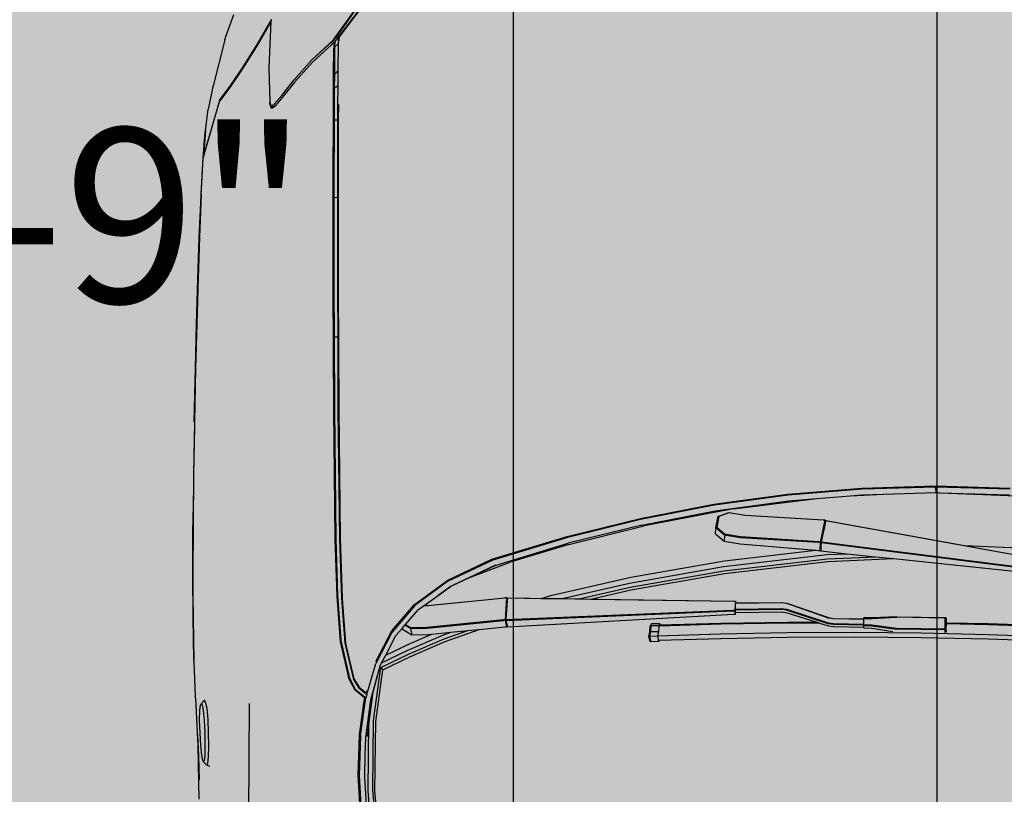
# Model space of a CAD drawing. Units: inches. Extents: x 1884 to 2398, y 474 to 1488.
# Tile 15 of 39: x 2186 to 2233, y 699 to 736. Entities that reach past the tile are written whole.
import ezdxf

# ---------------------------------------------------------------- set-up
doc = ezdxf.new("R2010")
doc.units = ezdxf.units.IN
doc.header["$MEASUREMENT"] = 0
doc.layers.get('0').update_dxf_attribs({"color": 250})
for name, color, linetype, lineweight in [('A-ANNO-DIMS', 2, 'Continuous', 18), ('A-AREA-IDEN', 7, 'Continuous', 18), ('C-VEHI', 8, 'Continuous', 18)]:
    doc.layers.add(name, color=color, linetype=linetype, lineweight=lineweight)
doc.layers.add('Edges', color=250, linetype='Continuous')
doc.layers.add('L-PVMT-PATT', color=9, linetype='Continuous', lineweight=13, true_color=0xc7c8ca)
doc.styles.get("Standard").update_dxf_attribs({"font": 'arial.ttf'})
doc.dimstyles.get("Standard").update_dxf_attribs({"dimtxt": 7, "dimasz": 0.18, "dimexe": 0.18, "dimexo": 0.0625, "dimgap": 0.09, "dimtad": 0, "dimtih": 1, "dimtoh": 1, "dimzin": 0, "dimdsep": 46, "dimlunit": 3, "dimtxsty": 'Standard', "dimcen": 0.09, "dimadec": 0, "dimazin": 0, "dimtfac": 1, "dimtofl": 0, "dimtmove": 0, "dimatfit": 3, "dimfxl": 1, "dimtolj": 1, "dimtzin": 0, "dimarcsym": 0})

# ---------------------------------------------------------------- blocks, each defined once
blk = doc.blocks.new('Nissan Qashqai pl')
at = {"layer": 'Edges'}
for p, q in [((8.4387, 12.0674), (8.4359, 11.9861)), ((8.4397, 12.0674), (8.4369, 11.9861)), ((8.4517, 12.0674), (8.4489, 11.9858)), ((8.4541, 11.9857), (8.4568, 12.0669)), ((8.3406, 11.9567), (8.3448, 12.0536)), ((8.3575, 12.0475), (8.3104, 11.7881)), ((8.336, 11.7828), (8.3688, 12.0419)), ((8.3702, 12.0427), (8.3374, 11.7826)), ((8.3565, 11.8707), (8.3746, 12.0435)), ((8.2765, 11.9273), (8.2804, 12.0305)), ((8.2682, 11.9221), (8.2708, 12.0123)), ((8.2719, 12.0118), (8.2695, 11.9221)), ((8.2765, 11.9273), (8.2788, 12.0114)), ((8.3406, 11.9567), (8.3495, 12.0053)), ((8.4359, 11.9861), (8.4348, 11.9346)), ((8.4369, 11.9861), (8.4358, 11.9346)), ((8.4489, 11.9858), (8.4471, 11.9043)), ((8.4523, 11.9043), (8.4541, 11.9857)), ((8.31, 11.7882), (8.3406, 11.9567)), ((8.4272, 11.8746), (8.4281, 11.9336)), ((8.4287, 11.9335), (8.4278, 11.8745)), ((8.4281, 11.9336), (8.429, 11.9345)), ((8.4281, 11.9336), (8.4287, 11.9336)), ((8.4287, 11.9335), (8.4281, 11.9336)), ((8.429, 11.9345), (8.4287, 11.9336)), ((8.4287, 11.9336), (8.4287, 11.9335)), ((8.4418, 11.9332), (8.4287, 11.9335)), ((8.4328, 11.9347), (8.429, 11.9345)), ((8.429, 11.9345), (8.4326, 11.9345)), ((8.4328, 11.9347), (8.4326, 11.9345)), ((8.4326, 11.9345), (8.4348, 11.9344)), ((8.4348, 11.9346), (8.4328, 11.9347)), ((8.4348, 11.9346), (8.4348, 11.9344)), ((8.4358, 11.9346), (8.4348, 11.9346)), ((8.4348, 11.9344), (8.4358, 11.9344)), ((8.4358, 11.9346), (8.4358, 11.9344)), ((8.4459, 11.9344), (8.4358, 11.9346)), ((8.4358, 11.9344), (8.4422, 11.9342)), ((8.441, 11.8742), (8.4418, 11.9332)), ((8.4418, 11.9332), (8.4422, 11.9342)), ((8.4431, 11.9332), (8.4418, 11.9332)), ((8.4422, 11.9342), (8.4459, 11.9344)), ((8.4422, 11.9342), (8.4431, 11.9332)), ((8.4431, 11.9332), (8.4422, 11.8742)), ((8.4464, 11.9334), (8.4431, 11.9332)), ((8.4459, 11.9344), (8.4459, 11.9344)), ((8.2708, 11.8319), (8.2682, 11.9221)), ((8.2763, 11.9223), (8.2695, 11.9221)), ((8.2695, 11.9221), (8.2763, 11.9219)), ((8.2695, 11.9221), (8.2719, 11.8323)), ((8.2763, 11.9223), (8.2764, 11.9263)), ((8.2763, 11.9219), (8.2763, 11.9223)), ((8.2781, 11.8585), (8.2763, 11.9219)), ((8.2764, 11.9263), (8.2765, 11.9273)), ((8.4471, 11.9043), (8.4464, 11.8227)), ((8.4516, 11.823), (8.4523, 11.9043)), ((8.3542, 11.8485), (8.3565, 11.8707)), ((8.3599, 11.7906), (8.3565, 11.8707)), ((8.4272, 11.8746), (8.4286, 11.8445)), ((8.4292, 11.8445), (8.4278, 11.8745)), ((8.4368, 11.8443), (8.441, 11.8742)), ((8.438, 11.8443), (8.4422, 11.8742)), ((8.4408, 11.8444), (8.4452, 11.8698)), ((8.28, 11.818), (8.2781, 11.8585)), ((8.2788, 11.8327), (8.2781, 11.8585)), ((8.2789, 11.8319), (8.2781, 11.8585)), ((8.3505, 11.8139), (8.3542, 11.8485)), ((8.3567, 11.7903), (8.3542, 11.8485)), ((8.4286, 11.8445), (8.4285, 11.8345)), ((8.4291, 11.8345), (8.4292, 11.8445)), ((8.4366, 11.8345), (8.4368, 11.8443)), ((8.4379, 11.8345), (8.438, 11.8443)), ((8.4406, 11.8344), (8.4408, 11.8444)), ((8.2781, 11.7423), (8.2708, 11.8319)), ((8.2719, 11.8323), (8.2793, 11.7426)), ((8.2789, 11.8319), (8.2788, 11.8327)), ((8.28, 11.818), (8.2789, 11.8319)), ((8.4291, 11.8345), (8.4285, 11.8345)), ((8.4298, 11.8345), (8.4291, 11.8345)), ((8.4292, 11.7978), (8.4298, 11.8345)), ((8.4304, 11.8345), (8.4298, 11.7978)), ((8.4304, 11.8345), (8.4298, 11.8345)), ((8.436, 11.8344), (8.4304, 11.8345)), ((8.4355, 11.7977), (8.436, 11.8344)), ((8.4366, 11.8343), (8.436, 11.8344)), ((8.4366, 11.8345), (8.4379, 11.8345)), ((8.4366, 11.8344), (8.4366, 11.8345)), ((8.4373, 11.8344), (8.4366, 11.8344)), ((8.4373, 11.8344), (8.4366, 11.8343)), ((8.4366, 11.8343), (8.4366, 11.8344)), ((8.4373, 11.8344), (8.4367, 11.7977)), ((8.4379, 11.8344), (8.4373, 11.8344)), ((8.4379, 11.8343), (8.4373, 11.8344)), ((8.4379, 11.8344), (8.4379, 11.8345)), ((8.4397, 11.8344), (8.4379, 11.8343)), ((8.4379, 11.8343), (8.4379, 11.8344)), ((8.4391, 11.7978), (8.4397, 11.8344)), ((8.4406, 11.8344), (8.4397, 11.8344)), ((8.452, 11.7418), (8.4516, 11.823)), ((8.2834, 11.7773), (8.28, 11.818)), ((8.3472, 11.7821), (8.3505, 11.8139)), ((8.3516, 11.79), (8.3505, 11.8139)), ((8.4464, 11.8227), (8.4468, 11.7413)), ((8.3092, 11.7863), (8.3093, 11.7873)), ((8.3093, 11.7873), (8.3367, 11.7816)), ((8.3159, 11.7869), (8.3093, 11.7873)), ((8.31, 11.7882), (8.3104, 11.7881)), ((8.3104, 11.7881), (8.3159, 11.7869)), ((8.3159, 11.7869), (8.336, 11.7828)), ((8.3662, 11.6639), (8.3516, 11.79)), ((8.3713, 11.6645), (8.3567, 11.7903)), ((8.3745, 11.665), (8.3599, 11.7906)), ((8.4107, 11.7411), (8.4281, 11.7914)), ((8.4287, 11.7914), (8.4111, 11.741)), ((8.4179, 11.7406), (8.4344, 11.7912)), ((8.4357, 11.7912), (8.4193, 11.7407)), ((8.4281, 11.7914), (8.4292, 11.7978)), ((8.4298, 11.7978), (8.4287, 11.7914)), ((8.4344, 11.7912), (8.4355, 11.7977)), ((8.4347, 11.7805), (8.4381, 11.7914)), ((8.4367, 11.7977), (8.4357, 11.7912)), ((8.4381, 11.7914), (8.4391, 11.7978)), ((8.296, 11.6762), (8.2834, 11.7773)), ((8.2862, 11.7434), (8.2834, 11.7773)), ((8.3038, 11.6903), (8.3095, 11.7853)), ((8.3099, 11.7851), (8.3042, 11.6901)), ((8.3092, 11.7863), (8.3099, 11.7851)), ((8.3095, 11.7853), (8.3092, 11.7863)), ((8.3298, 11.6848), (8.3355, 11.7798)), ((8.3369, 11.7796), (8.3312, 11.6846)), ((8.3355, 11.7798), (8.3366, 11.7806)), ((8.336, 11.7828), (8.3374, 11.7826)), ((8.3367, 11.7816), (8.3366, 11.7806)), ((8.3366, 11.7806), (8.3369, 11.7796)), ((8.3367, 11.7816), (8.347, 11.7811)), ((8.3374, 11.7826), (8.3406, 11.7824)), ((8.3385, 11.6842), (8.3464, 11.7761)), ((8.3458, 11.7813), (8.3406, 11.7824)), ((8.3406, 11.7824), (8.3457, 11.7821)), ((8.3458, 11.7813), (8.3457, 11.7821)), ((8.3457, 11.7821), (8.3472, 11.7821)), ((8.347, 11.7811), (8.3458, 11.7813)), ((8.3464, 11.7761), (8.3467, 11.7791)), ((8.3593, 11.6651), (8.3464, 11.7761)), ((8.3467, 11.7791), (8.347, 11.7811)), ((8.4222, 11.7413), (8.4337, 11.7775)), ((8.4337, 11.7775), (8.4347, 11.7805)), ((8.4337, 11.7775), (8.4339, 11.7423)), ((8.4347, 11.7805), (8.4348, 11.7421)), ((8.2905, 11.6524), (8.2781, 11.7423)), ((8.2793, 11.7426), (8.2916, 11.6528)), ((8.2985, 11.654), (8.2862, 11.7434)), ((8.4097, 11.7348), (8.4107, 11.7411)), ((8.4111, 11.741), (8.41, 11.7346)), ((8.417, 11.7342), (8.4179, 11.7406)), ((8.4193, 11.7407), (8.4183, 11.7343)), ((8.4213, 11.735), (8.4222, 11.7413)), ((8.4339, 11.7423), (8.4353, 11.6613)), ((8.4348, 11.7421), (8.4362, 11.661)), ((8.4468, 11.7413), (8.4482, 11.66)), ((8.4534, 11.6608), (8.452, 11.7418)), ((8.4104, 11.6791), (8.4097, 11.7348)), ((8.41, 11.7346), (8.4108, 11.6791)), ((8.4177, 11.678), (8.417, 11.7342)), ((8.4183, 11.7343), (8.4191, 11.678)), ((8.4221, 11.6787), (8.4213, 11.735)), ((8.3005, 11.6706), (8.3038, 11.6903)), ((8.3042, 11.6901), (8.3009, 11.6704)), ((8.3264, 11.6652), (8.3298, 11.6848)), ((8.3312, 11.6846), (8.3278, 11.665)), ((8.3352, 11.6646), (8.3385, 11.6842)), ((8.296, 11.6762), (8.3166, 11.5675)), ((8.3053, 11.6574), (8.3005, 11.6706)), ((8.3009, 11.6704), (8.3054, 11.6583)), ((8.4086, 11.6764), (8.4045, 11.4011)), ((8.4056, 11.5028), (8.4082, 11.6766)), ((8.4082, 11.6785), (8.4104, 11.6791)), ((8.4082, 11.6785), (8.4086, 11.6784)), ((8.4082, 11.6766), (8.4082, 11.6785)), ((8.4086, 11.6784), (8.4086, 11.6764)), ((8.4086, 11.6784), (8.4117, 11.6782)), ((8.4104, 11.6791), (8.4108, 11.6791)), ((8.4104, 11.6786), (8.4104, 11.6791)), ((8.4108, 11.6786), (8.4104, 11.6786)), ((8.4104, 11.6786), (8.4108, 11.6784)), ((8.4108, 11.6791), (8.4108, 11.6786)), ((8.4108, 11.6786), (8.4108, 11.6784)), ((8.4108, 11.6784), (8.4117, 11.6783)), ((8.4117, 11.6783), (8.4117, 11.6782)), ((8.4117, 11.6783), (8.4177, 11.678)), ((8.4117, 11.6782), (8.419, 11.6778)), ((8.4177, 11.678), (8.4191, 11.678)), ((8.419, 11.6778), (8.4203, 11.6778)), ((8.419, 11.6758), (8.419, 11.6778)), ((8.4305, 11.3996), (8.419, 11.6758)), ((8.4191, 11.678), (8.4221, 11.6787)), ((8.4238, 11.6786), (8.4203, 11.6778)), ((8.4203, 11.6778), (8.4204, 11.6758)), ((8.4204, 11.6758), (8.4319, 11.3996)), ((8.4238, 11.6786), (8.4221, 11.6787)), ((8.4238, 11.6766), (8.4238, 11.6786)), ((8.4394, 11.4014), (8.4238, 11.6766)), ((8.3054, 11.6583), (8.3053, 11.6574)), ((8.319, 11.6546), (8.3053, 11.6574)), ((8.3054, 11.6583), (8.3182, 11.6557)), ((8.3182, 11.6557), (8.3264, 11.6652)), ((8.319, 11.6546), (8.3182, 11.6557)), ((8.3278, 11.665), (8.319, 11.6546)), ((8.3264, 11.6542), (8.3352, 11.6646)), ((8.3278, 11.665), (8.3352, 11.6646)), ((8.3792, 11.5515), (8.3593, 11.6651)), ((8.3864, 11.5497), (8.3662, 11.6639)), ((8.3913, 11.5506), (8.3713, 11.6645)), ((8.3945, 11.5513), (8.3745, 11.665)), ((8.4353, 11.6613), (8.4375, 11.5863)), ((8.4362, 11.661), (8.4385, 11.5858)), ((8.4482, 11.66), (8.4505, 11.5843)), ((8.4557, 11.5855), (8.4534, 11.6608)), ((8.3076, 11.5631), (8.2905, 11.6524)), ((8.2916, 11.6528), (8.3089, 11.5631)), ((8.3157, 11.5647), (8.2985, 11.654)), ((8.3264, 11.6542), (8.319, 11.6546)), ((8.4377, 11.5857), (8.4357, 11.5864)), ((8.4357, 11.5864), (8.4359, 11.5765)), ((8.4357, 11.5864), (8.4375, 11.5863)), ((8.4375, 11.5863), (8.4375, 11.5862)), ((8.4379, 11.5758), (8.4377, 11.5857)), ((8.445, 11.5853), (8.4377, 11.5857)), ((8.4452, 11.5754), (8.445, 11.5853)), ((8.4503, 11.5841), (8.445, 11.5853)), ((8.4572, 11.5854), (8.4503, 11.5841)), ((8.4505, 11.5742), (8.4503, 11.5841)), ((8.4557, 11.5855), (8.4572, 11.5854)), ((8.4557, 11.5853), (8.4557, 11.5855)), ((8.4572, 11.5854), (8.4574, 11.5755)), ((8.4359, 11.5765), (8.4379, 11.5758)), ((8.4359, 11.5765), (8.4377, 11.5753)), ((8.4387, 11.5749), (8.4377, 11.5753)), ((8.4379, 11.5758), (8.4452, 11.5754)), ((8.4384, 11.5752), (8.4457, 11.5749)), ((8.446, 11.5746), (8.4387, 11.5749)), ((8.4452, 11.5754), (8.4505, 11.5742)), ((8.4507, 11.5734), (8.446, 11.5746)), ((8.4505, 11.5742), (8.4574, 11.5755)), ((8.4507, 11.5734), (8.4505, 11.5742)), ((8.4559, 11.5744), (8.4507, 11.5734)), ((8.4574, 11.5755), (8.4559, 11.5744)), ((8.3296, 11.4739), (8.3076, 11.5631)), ((8.3089, 11.5631), (8.3311, 11.4733)), ((8.3157, 11.5647), (8.3377, 11.4753)), ((8.3392, 11.4758), (8.3166, 11.5675)), ((8.4009, 11.4559), (8.3792, 11.5515)), ((8.4051, 11.4678), (8.3864, 11.5497)), ((8.4054, 11.4887), (8.3913, 11.5506)), ((8.4056, 11.5028), (8.3945, 11.5513)), ((8.4054, 11.4887), (8.4056, 11.5028)), ((8.4051, 11.4678), (8.4054, 11.4887)), ((8.3392, 11.4758), (8.3608, 11.4048)), ((8.3573, 11.3824), (8.3296, 11.4739)), ((8.3311, 11.4733), (8.3582, 11.3836)), ((8.3648, 11.3863), (8.3377, 11.4753)), ((8.4048, 11.4423), (8.4051, 11.4678)), ((8.4048, 11.4423), (8.4009, 11.4559)), ((8.4041, 11.4013), (8.4048, 11.4423)), ((8.3799, 11.3545), (8.3608, 11.4048)), ((8.407, 11.401), (8.4037, 11.4002)), ((8.4037, 11.4002), (8.4314, 11.3985)), ((8.4037, 11.3992), (8.4037, 11.4002)), ((8.4037, 11.3992), (8.4046, 11.3981)), ((8.4042, 11.3983), (8.4037, 11.3992)), ((8.4041, 11.4013), (8.4045, 11.4011)), ((8.4134, 11.3049), (8.4042, 11.3983)), ((8.4045, 11.4011), (8.407, 11.401)), ((8.4046, 11.3981), (8.4138, 11.3048)), ((8.407, 11.401), (8.4305, 11.3996)), ((8.4305, 11.3996), (8.4319, 11.3996)), ((8.4306, 11.3966), (8.4314, 11.3975)), ((8.4398, 11.3032), (8.4306, 11.3966)), ((8.4314, 11.3985), (8.4394, 11.4004)), ((8.4314, 11.3985), (8.4314, 11.3975)), ((8.4314, 11.3975), (8.4319, 11.3967)), ((8.4319, 11.3996), (8.436, 11.4006)), ((8.4319, 11.3967), (8.4412, 11.3033)), ((8.436, 11.4006), (8.4394, 11.4014)), ((8.4394, 11.4004), (8.436, 11.4006)), ((8.4394, 11.3984), (8.4394, 11.4004)), ((8.4425, 11.3672), (8.4394, 11.3984)), ((8.3826, 11.3291), (8.3573, 11.3824)), ((8.3582, 11.3836), (8.3844, 11.3284)), ((8.3646, 11.387), (8.3799, 11.3545)), ((8.3888, 11.3355), (8.3648, 11.3863)), ((8.4571, 11.3258), (8.4425, 11.3672)), ((8.4439, 11.3531), (8.4425, 11.3672)), ((8.3799, 11.3545), (8.3888, 11.3355)), ((8.454, 11.3245), (8.4439, 11.3531)), ((8.4459, 11.3326), (8.4439, 11.3531)), ((8.3901, 11.3328), (8.3888, 11.3355)), ((8.3901, 11.3328), (8.4011, 11.3173)), ((8.3904, 11.3321), (8.3901, 11.3328)), ((8.4011, 11.3173), (8.3904, 11.3321)), ((8.4493, 11.3229), (8.4459, 11.3326)), ((8.4482, 11.3095), (8.4459, 11.3326)), ((8.4122, 11.2883), (8.3826, 11.3291)), ((8.3844, 11.3284), (8.4134, 11.2888)), ((8.468, 11.2793), (8.4493, 11.3229)), ((8.4725, 11.2812), (8.454, 11.3245)), ((8.4756, 11.2826), (8.4571, 11.3258)), ((8.4135, 11.3), (8.4011, 11.3173)), ((8.4594, 11.2831), (8.4482, 11.3095)), ((8.4487, 11.305), (8.4482, 11.3095)), ((8.4135, 11.3), (8.4134, 11.3049)), ((8.4139, 11.2994), (8.4135, 11.3)), ((8.4138, 11.3048), (8.4139, 11.2994)), ((8.4183, 11.2934), (8.4139, 11.2994)), ((8.44, 11.2834), (8.4398, 11.3032)), ((8.4412, 11.3033), (8.4415, 11.2835)), ((8.4489, 11.2852), (8.4487, 11.305)), ((8.4444, 11.2608), (8.4122, 11.2883)), ((8.4134, 11.2888), (8.4462, 11.2609)), ((8.4365, 11.2776), (8.4183, 11.2934)), ((8.4415, 11.2835), (8.4489, 11.2852)), ((8.4422, 11.2737), (8.4489, 11.2852)), ((8.4365, 11.2776), (8.44, 11.2834)), ((8.4375, 11.2767), (8.4365, 11.2776)), ((8.4415, 11.2835), (8.4375, 11.2767)), ((8.4412, 11.2735), (8.4375, 11.2767)), ((8.4422, 11.2737), (8.4412, 11.2735)), ((8.4499, 11.2659), (8.4412, 11.2735)), ((8.4737, 11.2534), (8.4594, 11.2831)), ((8.4831, 11.2484), (8.468, 11.2793)), ((8.4889, 11.2473), (8.4725, 11.2812)), ((8.4914, 11.25), (8.4756, 11.2826)), ((8.4814, 11.2413), (8.4444, 11.2608)), ((8.4462, 11.2609), (8.4838, 11.2415)), ((8.4737, 11.2534), (8.4499, 11.2659)), ((8.4831, 11.2484), (8.4737, 11.2534)), ((8.4867, 11.2465), (8.4831, 11.2484)), ((8.4889, 11.2473), (8.4914, 11.25)), ((8.5544, 11.2416), (8.4914, 11.25)), ((8.7491, 11.2501), (8.6386, 11.2404)), ((8.5216, 11.2303), (8.4838, 11.2415)), ((8.528, 11.2354), (8.4867, 11.2465)), ((8.5214, 11.2374), (8.4867, 11.2465)), ((8.5531, 11.2387), (8.4889, 11.2473)), ((8.5214, 11.2374), (8.555, 11.233)), ((8.5301, 11.2352), (8.5214, 11.2374)), ((8.6375, 11.2376), (8.5531, 11.2387)), ((8.6386, 11.2404), (8.5544, 11.2416)), ((8.7481, 11.2473), (8.6375, 11.2376)), ((7.7261, 11.1898), (7.6762, 11.2256)), ((7.6762, 11.2256), (7.7233, 11.1928)), ((7.6769, 11.2312), (7.7194, 11.1992)), ((7.7232, 11.1955), (7.6771, 11.2307)), ((8.5125, 11.221), (8.5177, 11.2272)), ((8.5132, 11.2202), (8.5216, 11.2303)), ((8.5155, 11.2168), (8.5258, 11.2291)), ((8.5237, 11.2252), (8.5163, 11.2162)), ((8.5197, 11.2297), (8.5166, 11.2307)), ((8.5177, 11.2272), (8.5197, 11.2297)), ((8.5216, 11.2303), (8.5197, 11.2297)), ((8.5216, 11.2303), (8.5258, 11.2291)), ((8.5259, 11.2279), (8.5237, 11.2252)), ((8.5258, 11.2291), (8.5259, 11.2279)), ((8.5715, 11.2227), (8.5258, 11.2291)), ((8.5294, 11.2274), (8.5259, 11.2279)), ((8.5736, 11.2291), (8.528, 11.2354)), ((8.5706, 11.2216), (8.5294, 11.2274)), ((8.6387, 11.2319), (8.555, 11.233)), ((8.555, 11.233), (8.5726, 11.2307)), ((8.5941, 11.2286), (8.5736, 11.2291)), ((8.5941, 11.2289), (8.5941, 11.2286)), ((8.622, 11.228), (8.5941, 11.2286)), ((8.6699, 11.231), (8.622, 11.228)), ((8.6721, 11.2348), (8.6387, 11.2319)), ((8.4588, 11.2036), (8.5032, 11.2141)), ((8.4595, 11.2047), (8.5025, 11.2148)), ((8.5155, 11.2168), (8.5018, 11.2098)), ((8.5025, 11.2148), (8.5125, 11.221)), ((8.5163, 11.2162), (8.5029, 11.2092)), ((8.5032, 11.2141), (8.5132, 11.2202)), ((8.6197, 11.2201), (8.5706, 11.2216)), ((8.5715, 11.2227), (8.6203, 11.2213)), ((8.6683, 11.2226), (8.6197, 11.2201)), ((8.6203, 11.2213), (8.6721, 11.2241)), ((8.4042, 11.1995), (8.4588, 11.2036)), ((8.4049, 11.2004), (8.4595, 11.2047)), ((8.5018, 11.2098), (8.4559, 11.1991)), ((8.5029, 11.2092), (8.4571, 11.1983)), ((7.7194, 11.1992), (7.7232, 11.1966)), ((7.7232, 11.1966), (7.7279, 11.1965)), ((7.7281, 11.1918), (7.7232, 11.1955)), ((7.7232, 11.1955), (7.7245, 11.1955)), ((7.7267, 11.1902), (7.7233, 11.1928)), ((7.7247, 11.1954), (7.7245, 11.1955)), ((7.7245, 11.1955), (7.7294, 11.1955)), ((7.7261, 11.1898), (7.7507, 11.1638)), ((7.7286, 11.1881), (7.7267, 11.1902)), ((7.7281, 11.1918), (7.7299, 11.1904)), ((7.7349, 11.1917), (7.7281, 11.1918)), ((7.753, 11.1648), (7.7281, 11.1918)), ((7.7294, 11.1955), (7.731, 11.1955)), ((7.7299, 11.1904), (7.7324, 11.1876)), ((7.7299, 11.1904), (7.7364, 11.1904)), ((7.731, 11.1955), (7.7349, 11.1917)), ((7.731, 11.1955), (7.764, 11.1953)), ((7.768, 11.1915), (7.7349, 11.1917)), ((7.7363, 11.1904), (7.7364, 11.1904)), ((7.7694, 11.1901), (7.7364, 11.1904)), ((7.764, 11.1953), (7.7636, 11.1957)), ((7.768, 11.1915), (7.764, 11.1953)), ((7.764, 11.1953), (7.7662, 11.1953)), ((7.7659, 11.1957), (7.7662, 11.1953)), ((7.7662, 11.1953), (7.7668, 11.1946)), ((7.7662, 11.1953), (7.7811, 11.1952)), ((7.7692, 11.1915), (7.768, 11.1915)), ((7.7694, 11.1901), (7.7687, 11.1908)), ((7.7844, 11.1913), (7.7692, 11.1915)), ((7.7707, 11.1901), (7.7694, 11.1901)), ((7.7851, 11.19), (7.7707, 11.1901)), ((7.7811, 11.1952), (7.7809, 11.1958)), ((7.7814, 11.1946), (7.7811, 11.1952)), ((7.7811, 11.1952), (7.7822, 11.1952)), ((7.7822, 11.1952), (7.7819, 11.1958)), ((7.7822, 11.1952), (7.8057, 11.195)), ((7.7844, 11.1913), (7.7822, 11.1952)), ((7.8078, 11.1911), (7.7844, 11.1913)), ((7.7846, 11.1909), (7.7851, 11.19)), ((7.8083, 11.1898), (7.7851, 11.19)), ((7.8048, 11.1959), (7.8233, 11.1958)), ((7.8057, 11.195), (7.8233, 11.195)), ((7.8233, 11.1911), (7.8078, 11.1911)), ((7.904, 11.1894), (7.8083, 11.1898)), ((7.8233, 11.195), (7.8233, 11.1958)), ((7.8233, 11.1958), (7.9014, 11.1955)), ((7.8233, 11.195), (7.902, 11.1947)), ((7.8233, 11.1911), (7.8233, 11.195)), ((7.8233, 11.1899), (7.8233, 11.1911)), ((7.9036, 11.1907), (7.8233, 11.1911)), ((7.9014, 11.1955), (7.9185, 11.1955)), ((7.902, 11.1947), (7.9183, 11.1947)), ((7.9176, 11.1908), (7.9036, 11.1907)), ((8.0276, 11.1896), (7.904, 11.1894)), ((7.9183, 11.1947), (7.9176, 11.1908)), ((8.0275, 11.1909), (7.9176, 11.1908)), ((7.9185, 11.1955), (7.9183, 11.1947)), ((7.9183, 11.1947), (8.0275, 11.1948)), ((7.9185, 11.1955), (8.0273, 11.1957)), ((8.0273, 11.1957), (8.1753, 11.1963)), ((8.0275, 11.1948), (8.0876, 11.1951)), ((8.0873, 11.1911), (8.0275, 11.1909)), ((8.1753, 11.1903), (8.0276, 11.1896)), ((8.0876, 11.1951), (8.0873, 11.1911)), ((8.1755, 11.1915), (8.0873, 11.1911)), ((8.0876, 11.1951), (8.1754, 11.1954)), ((8.1753, 11.1963), (8.3318, 11.198)), ((8.3324, 11.192), (8.1753, 11.1903)), ((8.1754, 11.1954), (8.332, 11.1971)), ((8.3324, 11.1931), (8.1755, 11.1915)), ((8.3318, 11.198), (8.4049, 11.2004)), ((8.332, 11.1971), (8.4042, 11.1995)), ((8.4014, 11.1953), (8.3324, 11.1931)), ((8.4022, 11.1943), (8.3324, 11.192)), ((8.4559, 11.1991), (8.4014, 11.1953)), ((8.4571, 11.1983), (8.4022, 11.1943)), ((7.7507, 11.1638), (7.7286, 11.1881)), ((7.7324, 11.1876), (7.7539, 11.1642)), ((7.753, 11.1648), (7.7772, 11.1431)), ((7.7748, 11.1423), (7.7507, 11.1638)), ((7.7539, 11.1642), (7.7772, 11.1431)), ((7.7938, 11.1271), (7.7748, 11.1423)), ((7.7772, 11.1431), (7.7959, 11.1281)), ((7.8045, 11.1179), (7.7938, 11.1271)), ((7.7959, 11.1281), (7.8062, 11.1192)), ((7.8072, 11.1141), (7.8045, 11.1179)), ((7.8087, 11.1159), (7.8062, 11.1192)), ((7.8062, 11.1192), (7.8066, 11.1188)), ((7.8066, 11.1188), (7.8096, 11.1148)), ((7.701, 11.1141), (7.7024, 11.1141)), ((7.7038, 11.1132), (7.7024, 11.1141)), ((7.7024, 11.1141), (7.7034, 11.114)), ((7.7034, 11.114), (7.7056, 11.1128)), ((7.7034, 11.114), (7.7608, 11.1112)), ((7.7325, 11.0966), (7.7038, 11.1132)), ((7.7056, 11.1128), (7.7341, 11.0963)), ((7.7608, 11.1112), (7.8014, 11.1124)), ((7.8014, 11.1124), (7.8022, 11.1126)), ((7.8022, 11.1126), (7.8072, 11.1141)), ((7.8037, 11.1126), (7.8022, 11.1126)), ((7.8096, 11.1148), (7.8037, 11.1126)), ((7.8072, 11.1141), (7.8087, 11.1159)), ((7.7591, 11.08), (7.7325, 11.0966)), ((7.7341, 11.0963), (7.7606, 11.0798)), ((8.5326, 11.0874), (8.6675, 11.0866)), ((7.7814, 11.065), (7.7591, 11.08)), ((7.7606, 11.0798), (7.7828, 11.0649)), ((7.7223, 11.059), (7.6953, 11.0688)), ((7.7262, 11.0581), (7.7223, 11.059)), ((7.7262, 11.0581), (7.7819, 11.0438)), ((7.797, 11.0534), (7.7814, 11.065)), ((7.7828, 11.0649), (7.7984, 11.0533)), ((7.797, 11.0534), (7.797, 11.0534)), ((7.7998, 11.0513), (7.797, 11.0534)), ((7.7984, 11.0533), (7.8007, 11.0516)), ((7.7998, 11.0513), (7.8676, 11.0318)), ((7.8007, 11.0516), (7.8002, 11.0517)), ((7.8007, 11.0516), (7.8012, 11.0513)), ((7.8681, 11.032), (7.8012, 11.0513)), ((7.7819, 11.0438), (7.7848, 11.043)), ((7.7848, 11.043), (7.8087, 11.038)), ((7.8087, 11.038), (7.8106, 11.0377)), ((7.8107, 11.0377), (7.8106, 11.0377)), ((7.8363, 11.0344), (7.8107, 11.0377)), ((7.8381, 11.0342), (7.8363, 11.0344)), ((7.8363, 11.0344), (7.8676, 11.0318)), ((7.87, 11.0315), (7.8381, 11.0342)), ((8.5283, 11.0336), (8.5287, 11.0329)), ((8.531, 11.0346), (8.5287, 11.0329)), ((8.5385, 11.0363), (8.531, 11.0346)), ((8.5518, 11.0375), (8.5385, 11.0363)), ((8.568, 11.0382), (8.5518, 11.0375)), ((8.5526, 11.0328), (8.5681, 11.0335)), ((8.5842, 11.0384), (8.568, 11.0382)), ((8.5681, 11.0335), (8.5836, 11.0337)), ((8.5836, 11.0337), (8.5957, 11.0334)), ((8.5974, 11.0381), (8.5842, 11.0384)), ((8.5957, 11.0334), (8.6017, 11.0328)), ((8.6049, 11.0373), (8.5974, 11.0381)), ((8.6073, 11.0362), (8.6032, 11.0321)), ((8.6073, 11.0362), (8.6049, 11.0373)), ((8.609, 11.0397), (8.6073, 11.0362)), ((7.8681, 11.032), (7.8676, 11.0318)), ((7.8681, 11.032), (7.869, 11.0317)), ((7.9137, 11.0292), (7.869, 11.0317)), ((7.9151, 11.029), (7.87, 11.0315)), ((7.9137, 11.0292), (7.9658, 11.027)), ((7.9668, 11.0268), (7.9151, 11.029)), ((7.9658, 11.027), (8.016, 11.0253)), ((8.0168, 11.0251), (7.9668, 11.0268)), ((8.016, 11.0253), (8.0713, 11.0237)), ((8.0718, 11.0235), (8.0168, 11.0251)), ((8.0713, 11.0237), (8.1249, 11.0223)), ((8.1251, 11.0222), (8.0718, 11.0235)), ((8.1249, 11.0223), (8.1901, 11.021)), ((8.1902, 11.0208), (8.1251, 11.0222)), ((8.1902, 11.021), (8.1938, 11.021)), ((8.4811, 11.0203), (8.5241, 11.022)), ((8.5259, 11.0221), (8.5241, 11.022)), ((8.5259, 11.0221), (8.5838, 11.0251)), ((8.5287, 11.0329), (8.5331, 11.0292)), ((8.5331, 11.0292), (8.5346, 11.0303)), ((8.5347, 11.0282), (8.5331, 11.0292)), ((8.5346, 11.0303), (8.5406, 11.0316)), ((8.5407, 11.0274), (8.5347, 11.0282)), ((8.5406, 11.0316), (8.5526, 11.0328)), ((8.5527, 11.0273), (8.5407, 11.0274)), ((8.5682, 11.0278), (8.5527, 11.0273)), ((8.5837, 11.0288), (8.5682, 11.0278)), ((8.5707, 11.0248), (8.5965, 11.0258)), ((8.5958, 11.0301), (8.5837, 11.0288)), ((8.5838, 11.0251), (8.6489, 11.0263)), ((8.5838, 11.0251), (8.5965, 11.0258)), ((8.6018, 11.0312), (8.5958, 11.0301)), ((8.5965, 11.0258), (8.6252, 11.0268)), ((8.6017, 11.0328), (8.6032, 11.0321)), ((8.6032, 11.0321), (8.6018, 11.0312)), ((8.1901, 11.021), (8.1938, 11.021)), ((8.1904, 11.0209), (8.1902, 11.0208)), ((8.1904, 11.0209), (8.2543, 11.0198)), ((8.1938, 11.021), (8.1954, 11.0209)), ((8.1954, 11.0209), (8.2544, 11.02)), ((8.2544, 11.0198), (8.2543, 11.0199)), ((8.2543, 11.0198), (8.2544, 11.0198)), ((8.2544, 11.02), (8.3166, 11.0193)), ((8.2544, 11.0198), (8.2556, 11.0198)), ((8.2556, 11.0198), (8.256, 11.0198)), ((8.256, 11.0198), (8.2561, 11.0198)), ((8.2561, 11.0198), (8.2693, 11.0197)), ((8.2693, 11.0197), (8.2694, 11.0197)), ((8.2694, 11.0197), (8.3098, 11.0192)), ((8.3098, 11.0192), (8.3163, 11.0192)), ((8.3663, 11.019), (8.3163, 11.0192)), ((8.3597, 11.019), (8.3163, 11.0192)), ((8.3166, 11.0193), (8.3764, 11.0191)), ((8.3602, 11.019), (8.3597, 11.019)), ((8.3608, 11.019), (8.3602, 11.019)), ((8.3663, 11.019), (8.3608, 11.019)), ((8.3663, 11.019), (8.3764, 11.0191)), ((8.3757, 11.019), (8.3663, 11.019)), ((8.4282, 11.0193), (8.3757, 11.019)), ((8.3764, 11.0191), (8.4069, 11.0192)), ((8.4069, 11.0192), (8.4219, 11.0196)), ((8.4069, 11.0192), (8.4292, 11.0193)), ((8.4799, 11.0202), (8.4282, 11.0193)), ((8.4292, 11.0193), (8.4799, 11.0202)), ((8.4811, 11.0203), (8.4799, 11.0202))]:
    blk.add_line(p, q, dxfattribs=at)
blk = doc.blocks.new('car')
blk.add_blockref('Nissan Qashqai pl', (-9.7433, -11.9151))
blk = doc.blocks.new('carr')
blk.add_blockref('car', (0.5124, -0.007))
blk = doc.blocks.new('*D44')
at = {"layer": 'A-ANNO-DIMS', "color": 0, "lineweight": -2, "transparency": 16777216}
for p, q in [((2209.755, 1247.822), (2209.755, 484.005)), ((2230.029, 1247.822), (2230.029, 484.005)), ((2209.935, 484.185), (2229.849, 484.185)), ((2230.029, 484.185), (2230.209, 484.185))]:
    blk.add_line(p, q, dxfattribs=at)
at = {"layer": 'A-ANNO-DIMS', "color": 0, "lineweight": 100, "transparency": 16777216}
for points in [[(2209.935, 484.215), (2209.935, 484.155), (2209.755, 484.185)], [(2229.849, 484.215), (2229.849, 484.155), (2230.029, 484.185)]]:
    blk.add_solid(points, dxfattribs=at)
at = {"layer": 'Defpoints', "color": 0, "lineweight": 100, "transparency": 16777216}
for p in [(2209.755, 1247.885), (2230.029, 1247.885), (2230.029, 484.185)]:
    blk.add_point(p, dxfattribs=at)
at = {"layer": 'A-ANNO-DIMS', "color": 0, "transparency": 16777216, "insert": (2247.429, 484.185), "char_height": 7, "attachment_point": 5}
blk.add_mtext('\\A1;1\'-8 1/2"', dxfattribs=at)

msp = doc.modelspace()

# ---------------------------------------------------------------- hatches: boundary and pattern name
at = {"layer": 'L-PVMT-PATT'}
h = msp.add_hatch(color=256, dxfattribs=at)
h.dxf.hatch_style = 1
h.paths.add_polyline_path([(2387.529, 769.966), (2351.529, 769.966), (2238.447, 769.966), (2238.447, 762.15), (2238.447, 754.445), (2126.529, 754.445), (2126.529, 676.183), (2134.868, 676.183), (2142.673, 676.183), (2142.673, 646.578), (2134.868, 646.578), (2126.529, 646.578), (2126.529, 640.17), (2387.529, 640.17)])
h.paths.add_polyline_path([(2387.529, 631.385), (2303.086, 631.385), (2303.086, 615.671), (2387.529, 615.671)])
h.paths.add_polyline_path([(2387.529, 640.17), (2126.529, 640.17), (2126.529, 631.385), (2387.529, 631.385)])
h.paths.add_polyline_path([(2393.529, 604.13), (2387.529, 604.13), (2387.529, 615.671), (2303.086, 615.671), (2303.086, 607.943), (2249.649, 607.943), (2126.529, 607.943), (2126.529, 533.885), (2393.529, 533.885)])
h.paths.add_polyline_path([(2257.825, 611.008), (2257.83, 611.337), (2257.915, 616.493), (2258.021, 621.805), (2258.146, 627.274), (2258.252, 631.385), (2126.529, 631.385), (2126.529, 611.008)])
h.paths.add_polyline_path([(2258.892, 611.285), (2258.888, 611.008), (2300.247, 611.008), (2300.247, 631.385), (2259.314, 631.385), (2259.206, 627.173), (2259.081, 621.72), (2258.976, 616.424)])

# ---------------------------------------------------------------- block references
at = {"layer": 'C-VEHI', "xscale": 39.37007874015748, "yscale": 39.37007874015748, "zscale": 39.37007874015748, "rotation": 270}
msp.add_blockref('carr', (2229.977, 676.232), dxfattribs=at)

# ---------------------------------------------------------------- texts
at = {"layer": 'A-AREA-IDEN'}
msp.add_text('21\'-9"X13\'-9"', height=8.34125, dxfattribs=at).set_placement((2130.533, 722.895))

# ---------------------------------------------------------------- dimensions: what is measured, and where the dimension line sits
at = {"layer": 'A-ANNO-DIMS'}
dim = msp.add_linear_dim(base=(2230.029, 484.185), p1=(2209.755, 1247.885), p2=(2230.029, 1247.885), dimstyle='Standard', override={"dimdec": 1, "dimlfac": 1, "dimrnd": 0, "dimzin": 1, "dimdsep": 46, "dimlunit": 4, "dimfrac": 2}, dxfattribs=at)
dim.commit()
dim.dimension.update_dxf_attribs({"geometry": '*D44', "text_midpoint": (2247.429, 484.185)})

doc.saveas('drawing.dxf')
